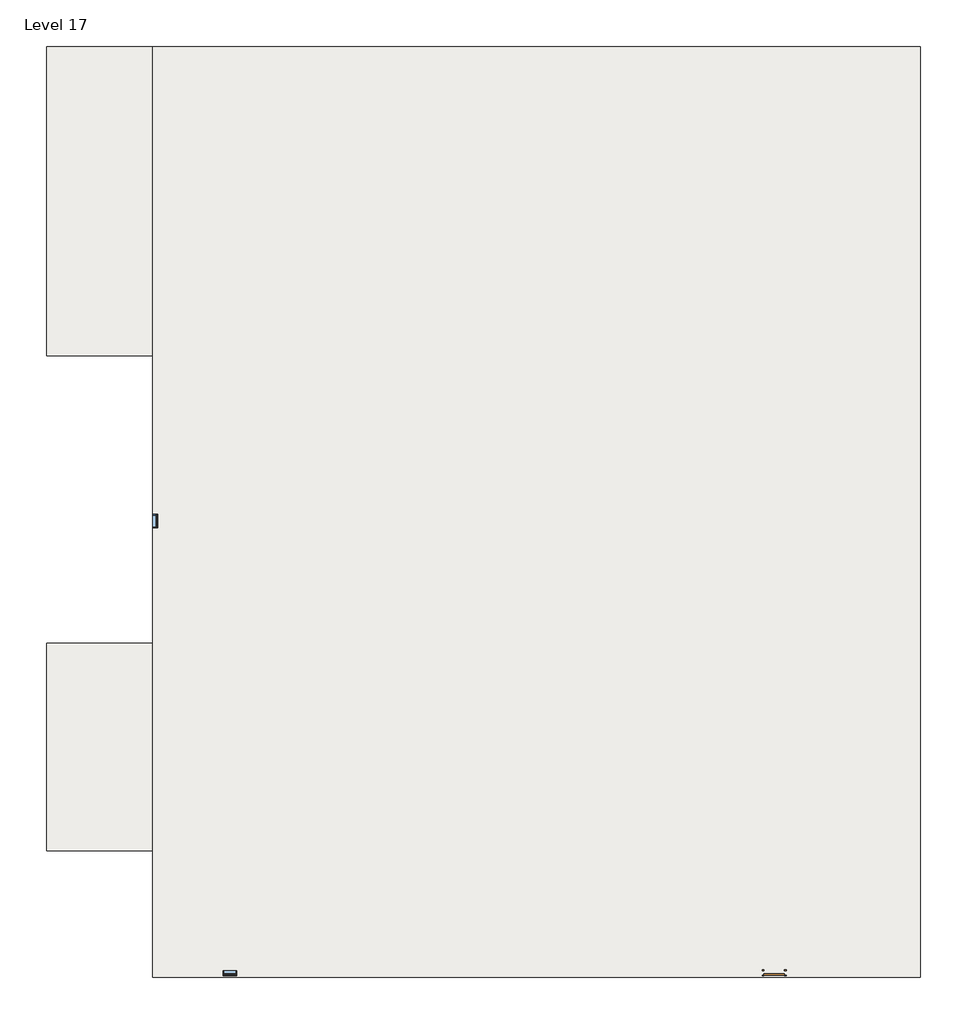
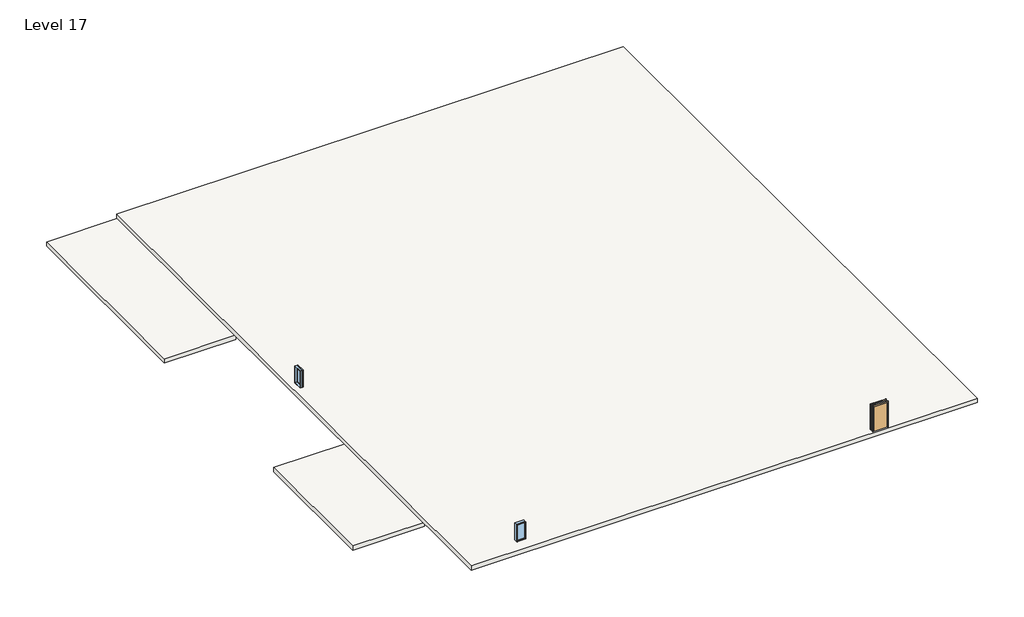
# One storey: 3 slabs, 2 windows, 1 door.
"""IFC4 building model written with IfcOpenShell, lengths in millimetres."""

from ifc_helpers import new_model, si_unit, frame, origin, place, context, project, spatial, polyline, outline, extrude, transform, mapped, element, save
from components import door_719f80de, window_80bd9af0, window_78885257

model = new_model("IFC4")

# Units and contexts
model_context = context("Model", 3, world=origin())
ifc_project = project(units=[si_unit("LENGTHUNIT", "METRE", prefix="MILLI")], contexts=[model_context])

# Site, building, storey
site = spatial("IfcSite", under=ifc_project)
building = spatial("IfcBuilding", under=site)
storey = spatial("IfcBuildingStorey", under=building, Name="Level 17", Elevation=29565.6)

# Door
placement = place(None, origin())
door_shape = door_719f80de(model_context)
element("IfcDoor", 1, ObjectType="Single-Flush : 36\" x 84\"", at=placement, inside=storey, context=model_context, shape_type="MappedRepresentation", body=[
    mapped(door_shape, transform((12612.561926, -20744.1985361, 29565.6), x_axis=(1.0, 0.0, 0.0), y_axis=(0.0, 1.0, 0.0), z_axis=(0.0, 0.0, 1.0))),
])

# Slabs
element("IfcSlab", 2, ObjectType="Generic - 12\"", at=placement, inside=storey, context=model_context, shape_type="SweptSolid", body=[
    extrude(outline(polyline([(19165.761926, 20806.0329695), (19165.761926, -20951.5670305), (-15276.638074, -20951.5670305), (-15276.638074, 20806.0329695), (19165.761926, 20806.0329695)])), frame((0.0, 0.0, 29603.7561104), z_axis=(0.0, 0.0, 1.0), x_axis=(1.0, 0.0, 0.0)), (0.0, 0.0, 1.0), 304.8),
])
element("IfcSlab", 3, ObjectType="Generic - 12\"", at=placement, inside=storey, context=model_context, shape_type="SweptSolid", body=[
    extrude(outline(polyline([(-20051.838074, -15263.2213044), (-20051.838074, -5966.8213044), (-15175.038074, -5966.8213044), (-15175.038074, -15263.2213044), (-20051.838074, -15263.2213044)])), frame((0.0, 0.0, 29260.8), z_axis=(0.0, 0.0, 1.0), x_axis=(1.0, 0.0, 0.0)), (0.0, 0.0, 1.0), 304.8),
])
element("IfcSlab", 4, ObjectType="Generic - 12\"", at=placement, inside=storey, context=model_context, shape_type="SweptSolid", body=[
    extrude(outline(polyline([(-20051.838074, 20810.2014639), (-15175.038074, 20810.2014639), (-15175.038074, 6941.8014639), (-20051.838074, 6941.8014639), (-20051.838074, 20810.2014639)])), frame((0.0, 0.0, 29260.8), z_axis=(0.0, 0.0, 1.0), x_axis=(1.0, 0.0, 0.0)), (0.0, 0.0, 1.0), 304.8),
])

# Windows
window_shape = window_80bd9af0(model_context)
element("IfcWindow", 5, ObjectType="Fixed : 24\" x 48\"", at=placement, inside=storey, context=model_context, shape_type="MappedRepresentation", body=[
    mapped(window_shape, transform((-15175.038074, -518.5213044, 29565.6), x_axis=(0.0, -1.0, 0.0), y_axis=(1.0, 0.0, 0.0), z_axis=(0.0, 0.0, 1.0))),
])
window_2_shape = window_78885257(model_context)
element("IfcWindow", 6, ObjectType="Instance - Fixed : 24\" x 48\"", at=placement, inside=storey, context=model_context, shape_type="MappedRepresentation", body=[
    mapped(window_2_shape, transform((-11860.338074, -20744.1985361, 29565.6), x_axis=(-1.0, 0.0, 0.0), y_axis=(0.0, -1.0, 0.0), z_axis=(0.0, 0.0, 1.0))),
])

save(model, "model.ifc")

# Revit data of these elements
# Type "Single-Flush : 36\" x 84\""
#   Type Mark = "1"
#   Construction Type Id = "MDOOR"
#   Assembly Code = "C1020"
#   Analytic Construction = "Metal"
#   Thickness = 0' - 2"
#   Heat Transfer Coefficient (U) = 0.651978 BTU/(h·ft²·°F)
#   Height = 7' - 0"
#   Trim Projection Ext = 0' - 1"
#   Trim Projection Int = 0' - 1"
#   Trim Width = 0' - 3"
#   Width = 3' - 0"
#   Define Thermal Properties by = 1
#   Door Material = Door - Panel
#   Frame Material = Door - Frame
#   Visual Light Transmittance = 0
#   Solar Heat Gain Coefficient = 0
#   Function = (empty or 0)
#   Wall Closure = (empty or 0)
# Type "Generic - 12\""
#   Assembly Code = "B1010"
#   Function = 0
#   Layers, outside or top first: 1' - 0" no material (function 1)
# Type "Fixed : 24\" x 48\""
#   Type Mark = "2"
#   Construction Type Id = "GSP4R"
#   Assembly Code = "B2020100"
#   Analytic Construction = "1/8 in Pilkington single glazing"
#   Visual Light Transmittance = 0.9
#   Solar Heat Gain Coefficient = 0.78
#   Heat Transfer Coefficient (U) = 0.6496 BTU/(h·ft²·°F)
#   Height = 4' - 0"
#   Default Sill Height = 3' - 0"
#   Width = 2' - 0"
#   Window Inset = 0' - 0 3/4"
#   Define Thermal Properties by = 1
#   Glass Pane Material = Glass
#   Sash Material = Sash
#   Wall Closure = (empty or 0)
# Type "Instance - Fixed : 24\" x 48\""
#   Type Mark = "19"
#   Construction Type Id = "GSP4R"
#   Assembly Code = "B2020100"
#   Analytic Construction = "1/8 in Pilkington single glazing"
#   Visual Light Transmittance = 0.9
#   Thermal Resistance (R) = 0.8466 (h·ft²·°F)/BTU
#   Solar Heat Gain Coefficient = 0.86
#   Heat Transfer Coefficient (U) = 1.1812 BTU/(h·ft²·°F)
#   Height [instance default] = 4' - 0"
#   Default Sill Height = 3' - 0"
#   Width [instance default] = 2' - 0"
#   Window Inset = 0' - 0 3/4"
#   Define Thermal Properties by = 1
#   Glass Pane Material = Glass
#   Sash Material = Sash
#   Wall Closure = (empty or 0)
# Element 1 (IfcDoor, "Single-Flush : 36\" x 84\"")
#   Phase Created = New Construction
#   Materials on its faces: "Door - Frame", "Door - Panel"
# Element 2 (IfcSlab, "Generic - 12\"")
#   Height Offset From Level = 1' - 1.50221"
#   Phase Created = New Construction
#   Materials on its faces: "Default Floor"
# Elements 3, 4 (IfcSlab, "Generic - 12\"")
#   built-in parameter 1001955 = 3.14159 (stored number, unit not read)
#   Height Offset From Level = 0' - 0"
#   Phase Created = New Construction
#   Materials on its faces: "Default Floor"
# Element 5 (IfcWindow, "Fixed : 24\" x 48\"")
#   Mark = "47"
#   Phase Created = New Construction
#   Materials on its faces: "Sash", "Glass"
# Element 6 (IfcWindow, "Instance - Fixed : 24\" x 48\"")
#   Mark = "14"
#   Width = 2' - 0"
#   Height = 4' - 0"
#   Phase Created = New Construction
#   Materials on its faces: "Sash", "Glass"
# Materials
#   "Door - Panel": class "Wood", colour RGB 210 159 95, transparency 0
#   "Door - Frame": colour RGB 118 70 51, transparency 0
#   "Glass": class "Glass", colour RGB 0 128 192, transparency 0.75, Description = "Soda Lime Glass", Cost = 0
#   "Sash": class "Wood", colour RGB 224 178 126, transparency 0
#   "Default Floor": colour RGB 128 128 128, transparency 0
